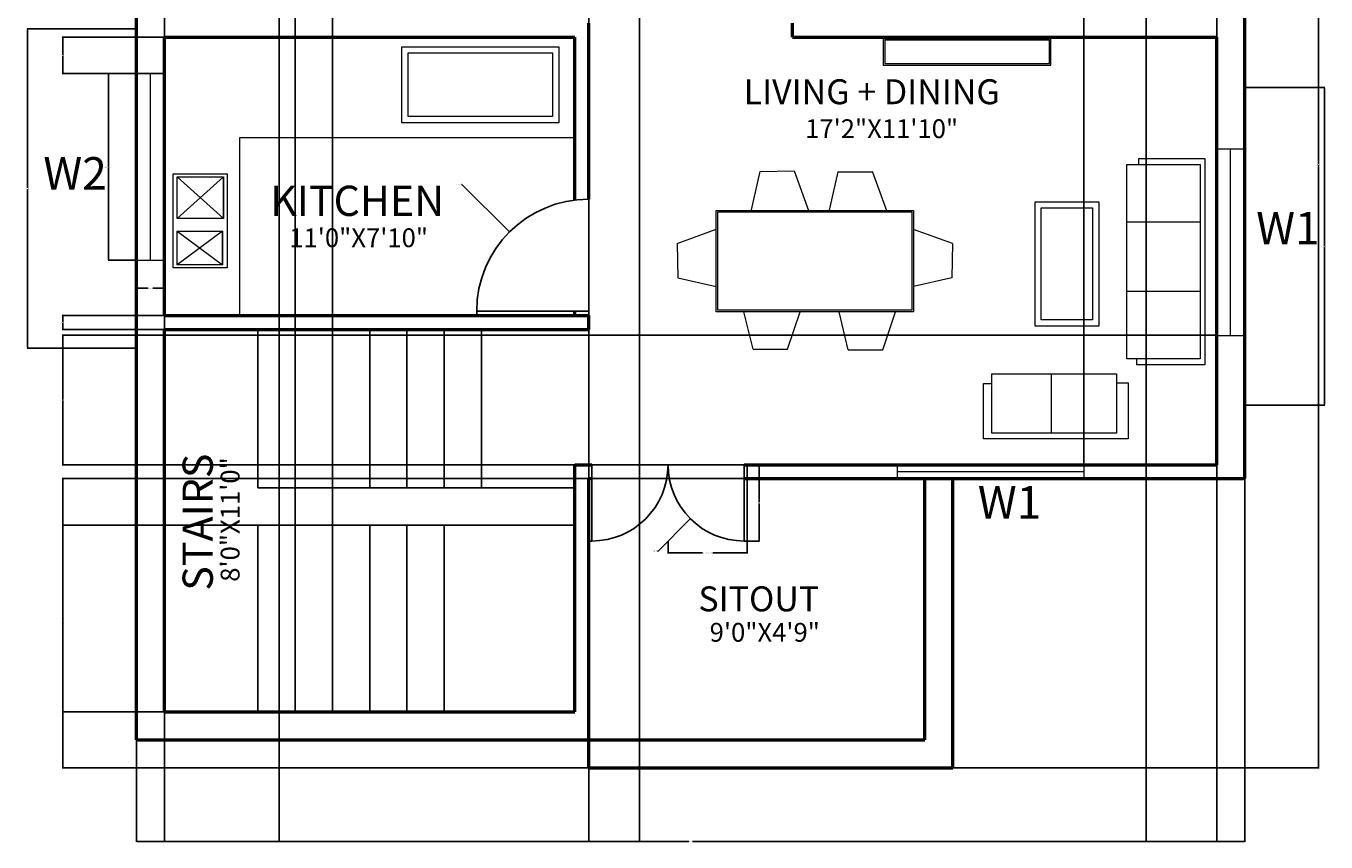
# Model space of a CAD drawing. Units: inches. Extents: x -26 to 394, y -29 to 465.
# Tile 1 of 2: x -26 to 392, y -29 to 234. Entities that reach past the tile are written whole.
import ezdxf

# ---------------------------------------------------------------- set-up
doc = ezdxf.new("R2010")
doc.units = ezdxf.units.IN
doc.header["$MEASUREMENT"] = 0
for name, color, linetype, lineweight, true_color in [('A-ANNO-DIMS', 254, 'Continuous', 18, 0xfeeab9), ('A-FLOR-FIXT', 254, 'Continuous', 18, 0xfeeab9), ('A-FURN', 254, 'Continuous', 18, 0xfeeab9)]:
    doc.layers.add(name, color=color, linetype=linetype, lineweight=lineweight, true_color=true_color)
for name, color, linetype, lineweight in [('A-ANNO-TEXT', 7, 'Continuous', 18), ('A-AREA-IDEN', 7, 'Continuous', 25), ('A-DOOR', 3, 'Continuous', 25), ('A-FLOR-STRS', 7, 'Continuous', 25), ('A-GLAZ', 4, 'Continuous', 18), ('A-WALL', 7, 'Continuous', 50)]:
    doc.layers.add(name, color=color, linetype=linetype, lineweight=lineweight)
doc.styles.get("Standard").update_dxf_attribs({"font": 'arial.ttf'})
doc.dimstyles.get("Standard").update_dxf_attribs({"dimtxt": 0.18, "dimasz": 0.18, "dimexe": 0.18, "dimexo": 0.0625, "dimgap": 0.09, "dimtad": 0, "dimtih": 1, "dimtoh": 1, "dimdec": 4, "dimzin": 0, "dimdsep": 46, "dimtxsty": 'Standard', "dimcen": 0.09, "dimadec": 0, "dimazin": 0, "dimtfac": 1, "dimtdec": 4, "dimtofl": 0, "dimtmove": 0, "dimatfit": 3, "dimfxl": 1, "dimtolj": 1, "dimtzin": 0, "dimarcsym": 0})

# ---------------------------------------------------------------- blocks, each defined once
blk = doc.blocks.new('*D10')
at = {"layer": 'A-ANNO-DIMS', "color": 0, "lineweight": -2, "transparency": 16777216}
for p, q in [((366.09, 214), (392.09, 214)), ((391.91, 213.82), (391.91, 163.15)), ((391.91, 112.11), (391.91, 162.79)), ((366.09, 111.93), (392.09, 111.93))]:
    blk.add_line(p, q, dxfattribs=at)
at = {"layer": 'A-ANNO-DIMS', "color": 0, "transparency": 16777216}
for points in [[(391.88, 213.82), (391.94, 213.82), (391.91, 214)], [(391.88, 112.11), (391.94, 112.11), (391.91, 111.93)]]:
    blk.add_solid(points, dxfattribs=at)
at = {"layer": 'Defpoints', "color": 0, "transparency": 16777216}
for p in [(366.02, 214), (366.02, 111.93), (391.91, 111.93)]:
    blk.add_point(p, dxfattribs=at)
at = {"layer": 'A-ANNO-DIMS', "color": 0, "transparency": 16777216, "insert": (391.91, 162.97), "char_height": 0.18, "attachment_point": 5}
blk.add_mtext('\\A1;102.0697', dxfattribs=at)
blk = doc.blocks.new('*D11')
at = {"layer": 'A-ANNO-DIMS', "color": 0, "lineweight": -2, "transparency": 16777216}
for p, q in [((9.7, 232.88), (-25.34, 232.88)), ((-25.16, 232.7), (-25.16, 181.74)), ((-25.16, 130.42), (-25.16, 181.38)), ((9.7, 130.24), (-25.34, 130.24))]:
    blk.add_line(p, q, dxfattribs=at)
at = {"layer": 'A-ANNO-DIMS', "color": 0, "transparency": 16777216}
for points in [[(-25.19, 232.7), (-25.13, 232.7), (-25.16, 232.88)], [(-25.19, 130.42), (-25.13, 130.42), (-25.16, 130.24)]]:
    blk.add_solid(points, dxfattribs=at)
at = {"layer": 'Defpoints', "color": 0, "transparency": 16777216}
for p in [(9.77, 232.88), (-25.16, 130.24), (9.77, 130.24)]:
    blk.add_point(p, dxfattribs=at)
at = {"layer": 'A-ANNO-DIMS', "color": 0, "transparency": 16777216, "insert": (-25.16, 181.56), "char_height": 0.18, "attachment_point": 5}
blk.add_mtext('\\A1;102.6356', dxfattribs=at)
blk = doc.blocks.new('WIN-60IN-9IN-JAMB')
for p, q in [((0, 9), (0, 0)), ((60, 9), (60, 0)), ((0, 4.5), (60, 4.5))]:
    blk.add_line(p, q)
blk = doc.blocks.new('DOOR-36IN-INTERIOR')
blk.add_lwpolyline([(0, 1.36), (0, 0), (36.04, 0), (36.04, 1.36)], close=True)
blk.add_arc((36, 1.36), 36, 90, 180)
blk = doc.blocks.new('DOOR-ENTRY-LEAF')
blk.add_lwpolyline([(24.53, 0), (25.46, 0), (25.46, 24.56), (24.53, 24.56)], close=True)
blk.add_arc((24.53, 24.53), 24.53, 180, 270)
blk = doc.blocks.new('FURN-WALL-UNIT')
for points in [[(8.48, 53.93), (0, 53.93), (0, 0), (8.48, 0)], [(7.98, 53.43), (0.5, 53.43), (0.5, 0.5), (7.98, 0.5)]]:
    blk.add_lwpolyline(points, close=True)
blk = doc.blocks.new('*D18')
at = {"layer": 'A-ANNO-DIMS', "color": 0, "lineweight": -2, "transparency": 16777216}
for p, q in [((9.84, 218.5), (0.72, 218.5)), ((0.9, 218.32), (0.9, 188.68)), ((0.9, 158.68), (0.9, 188.32)), ((9.84, 158.5), (0.72, 158.5))]:
    blk.add_line(p, q, dxfattribs=at)
at = {"layer": 'A-ANNO-DIMS', "color": 0, "transparency": 16777216}
for points in [[(0.87, 218.32), (0.93, 218.32), (0.9, 218.5)], [(0.87, 158.68), (0.93, 158.68), (0.9, 158.5)]]:
    blk.add_solid(points, dxfattribs=at)
at = {"layer": 'Defpoints', "color": 0, "transparency": 16777216}
for p in [(0.9, 218.5), (9.9, 218.5), (9.9, 158.5)]:
    blk.add_point(p, dxfattribs=at)
at = {"layer": 'A-ANNO-DIMS', "color": 0, "transparency": 16777216, "insert": (0.9, 188.5), "char_height": 0.18, "attachment_point": 5}
blk.add_mtext('\\A1;WINDOW 60.0000 TYP.', dxfattribs=at)
blk = doc.blocks.new('*D19')
at = {"layer": 'A-ANNO-DIMS', "color": 0, "lineweight": -2, "transparency": 16777216}
for p, q in [((9.9, 158.44), (9.9, 149.32)), ((18.9, 158.44), (18.9, 149.32)), ((10.08, 149.5), (13.63, 149.5)), ((18.72, 149.5), (15.17, 149.5))]:
    blk.add_line(p, q, dxfattribs=at)
at = {"layer": 'A-ANNO-DIMS', "color": 0, "transparency": 16777216}
for points in [[(10.08, 149.53), (10.08, 149.47), (9.9, 149.5)], [(18.72, 149.53), (18.72, 149.47), (18.9, 149.5)]]:
    blk.add_solid(points, dxfattribs=at)
at = {"layer": 'Defpoints', "color": 0, "transparency": 16777216}
for p in [(9.9, 158.5), (18.9, 158.5), (9.9, 149.5)]:
    blk.add_point(p, dxfattribs=at)
at = {"layer": 'A-ANNO-DIMS', "color": 0, "transparency": 16777216, "insert": (14.4, 149.5), "char_height": 0.18, "attachment_point": 5}
blk.add_mtext('\\A1;9.0000 TYP.', dxfattribs=at)
blk = doc.blocks.new('*D26')
at = {"layer": 'A-ANNO-DIMS', "color": 0, "lineweight": -2, "transparency": 16777216}
for p, q in [((180.81, 68.15), (180.81, 64.22)), ((206.27, 68.15), (206.27, 64.22)), ((180.99, 64.4), (191.89, 64.4)), ((206.09, 64.4), (195.19, 64.4))]:
    blk.add_line(p, q, dxfattribs=at)
at = {"layer": 'A-ANNO-DIMS', "color": 0, "transparency": 16777216}
for points in [[(180.99, 64.43), (180.99, 64.37), (180.81, 64.4)], [(206.09, 64.43), (206.09, 64.37), (206.27, 64.4)]]:
    blk.add_solid(points, dxfattribs=at)
at = {"layer": 'Defpoints', "color": 0, "transparency": 16777216}
for p in [(180.81, 68.21), (206.27, 68.21), (206.27, 64.4)]:
    blk.add_point(p, dxfattribs=at)
at = {"layer": 'A-ANNO-DIMS', "color": 0, "transparency": 16777216, "insert": (193.54, 64.4), "char_height": 0.18, "attachment_point": 5}
blk.add_mtext('\\A1;ENTRY LEAF 25.4567 TYP.', dxfattribs=at)
blk = doc.blocks.new('*D27')
at = {"layer": 'A-ANNO-DIMS', "color": 0, "lineweight": -2, "transparency": 16777216}
for p, q in [((206.33, 92.77), (210.27, 92.77)), ((210.09, 92.59), (210.09, 80.67)), ((210.09, 68.39), (210.09, 80.31)), ((206.33, 68.21), (210.27, 68.21))]:
    blk.add_line(p, q, dxfattribs=at)
at = {"layer": 'A-ANNO-DIMS', "color": 0, "transparency": 16777216}
for points in [[(210.06, 92.59), (210.12, 92.59), (210.09, 92.77)], [(210.06, 68.39), (210.12, 68.39), (210.09, 68.21)]]:
    blk.add_solid(points, dxfattribs=at)
at = {"layer": 'Defpoints', "color": 0, "transparency": 16777216}
for p in [(206.27, 92.77), (210.09, 92.77), (206.27, 68.21)]:
    blk.add_point(p, dxfattribs=at)
at = {"layer": 'A-ANNO-DIMS', "color": 0, "transparency": 16777216, "insert": (210.09, 80.49), "char_height": 0.18, "attachment_point": 5}
blk.add_mtext('\\A1;24.5570 TYP.', dxfattribs=at)
blk = doc.blocks.new('*D30')
at = {"layer": 'A-ANNO-DIMS', "color": 0, "lineweight": -2, "transparency": 16777216}
for p, q in [((366.35, 88.21), (366.35, -28.56)), ((9.85, 4.21), (9.85, -28.56)), ((10.03, -28.38), (187.5, -28.38)), ((366.17, -28.38), (188.71, -28.38))]:
    blk.add_line(p, q, dxfattribs=at)
at = {"layer": 'A-ANNO-DIMS', "color": 0, "transparency": 16777216}
for points in [[(10.03, -28.35), (10.03, -28.41), (9.85, -28.38)], [(366.17, -28.35), (366.17, -28.41), (366.35, -28.38)]]:
    blk.add_solid(points, dxfattribs=at)
at = {"layer": 'Defpoints', "color": 0, "transparency": 16777216}
for p in [(366.35, 88.27), (9.85, 4.27), (366.35, -28.38)]:
    blk.add_point(p, dxfattribs=at)
at = {"layer": 'A-ANNO-DIMS', "color": 0, "transparency": 16777216, "insert": (188.1, -28.38), "char_height": 0.18, "attachment_point": 5}
blk.add_mtext('\\A1;356.5000', dxfattribs=at)
blk = doc.blocks.new('*D31')
at = {"layer": 'A-ANNO-DIMS', "color": 0, "lineweight": -2, "transparency": 16777216}
for p, q in [((366.42, 383.27), (390.18, 383.27)), ((390, 383.09), (390, 189.45)), ((390, -4.55), (390, 189.09)), ((272.42, -4.73), (390.18, -4.73))]:
    blk.add_line(p, q, dxfattribs=at)
at = {"layer": 'A-ANNO-DIMS', "color": 0, "transparency": 16777216}
for points in [[(389.97, 383.09), (390.03, 383.09), (390, 383.27)], [(389.97, -4.55), (390.03, -4.55), (390, -4.73)]]:
    blk.add_solid(points, dxfattribs=at)
at = {"layer": 'Defpoints', "color": 0, "transparency": 16777216}
for p in [(366.35, 383.27), (390, 383.27), (272.35, -4.73)]:
    blk.add_point(p, dxfattribs=at)
at = {"layer": 'A-ANNO-DIMS', "color": 0, "transparency": 16777216, "insert": (390, 189.27), "char_height": 0.18, "attachment_point": 5}
blk.add_mtext('\\A1;388.0000', dxfattribs=at)
blk = doc.blocks.new('*D32')
at = {"layer": 'A-ANNO-DIMS', "color": 0, "lineweight": -2, "transparency": 16777216}
for p, q in [((272.29, 88.27), (-14.04, 88.27)), ((-13.86, 88.09), (-13.86, 41.95)), ((-13.86, -4.55), (-13.86, 41.59)), ((272.29, -4.73), (-14.04, -4.73))]:
    blk.add_line(p, q, dxfattribs=at)
at = {"layer": 'A-ANNO-DIMS', "color": 0, "transparency": 16777216}
for points in [[(-13.89, 88.09), (-13.83, 88.09), (-13.86, 88.27)], [(-13.89, -4.55), (-13.83, -4.55), (-13.86, -4.73)]]:
    blk.add_solid(points, dxfattribs=at)
at = {"layer": 'Defpoints', "color": 0, "transparency": 16777216}
for p in [(-13.86, 88.27), (272.35, 88.27), (272.35, -4.73)]:
    blk.add_point(p, dxfattribs=at)
at = {"layer": 'A-ANNO-DIMS', "color": 0, "transparency": 16777216, "insert": (-13.86, 41.77), "char_height": 0.18, "attachment_point": 5}
blk.add_mtext('\\A1;93.0000', dxfattribs=at)
blk = doc.blocks.new('*D34')
at = {"layer": 'A-ANNO-DIMS', "color": 0, "lineweight": -2, "transparency": 16777216}
for p, q in [((155.35, 374.21), (155.35, -28.56)), ((171.67, 374.21), (171.67, -28.56)), ((155.53, -28.38), (162.99, -28.38)), ((171.49, -28.38), (164.04, -28.38))]:
    blk.add_line(p, q, dxfattribs=at)
at = {"layer": 'A-ANNO-DIMS', "color": 0, "transparency": 16777216}
for points in [[(155.53, -28.35), (155.53, -28.41), (155.35, -28.38)], [(171.49, -28.35), (171.49, -28.41), (171.67, -28.38)]]:
    blk.add_solid(points, dxfattribs=at)
at = {"layer": 'Defpoints', "color": 0, "transparency": 16777216}
for p in [(155.35, 374.27), (171.67, 374.27), (171.67, -28.38)]:
    blk.add_point(p, dxfattribs=at)
at = {"layer": 'A-ANNO-DIMS', "color": 0, "transparency": 16777216, "insert": (163.51, -28.38), "char_height": 0.18, "attachment_point": 5}
blk.add_mtext('\\A1;16.3118', dxfattribs=at)
blk = doc.blocks.new('*D35')
at = {"layer": 'A-ANNO-DIMS', "color": 0, "lineweight": -2, "transparency": 16777216}
for p, q in [((314.49, 92.86), (314.49, 407.1)), ((314.67, 406.92), (335.38, 406.92)), ((357.17, 406.92), (336.46, 406.92)), ((357.35, 92.83), (357.35, 407.1))]:
    blk.add_line(p, q, dxfattribs=at)
at = {"layer": 'A-ANNO-DIMS', "color": 0, "transparency": 16777216}
for points in [[(314.67, 406.95), (314.67, 406.89), (314.49, 406.92)], [(357.17, 406.95), (357.17, 406.89), (357.35, 406.92)]]:
    blk.add_solid(points, dxfattribs=at)
at = {"layer": 'Defpoints', "color": 0, "transparency": 16777216}
for p in [(357.35, 406.92), (314.49, 92.8), (357.35, 92.77)]:
    blk.add_point(p, dxfattribs=at)
at = {"layer": 'A-ANNO-DIMS', "color": 0, "transparency": 16777216, "insert": (335.92, 406.92), "char_height": 0.18, "attachment_point": 5}
blk.add_mtext('\\A1;42.8686', dxfattribs=at)
blk = doc.blocks.new('*D36')
at = {"layer": 'A-ANNO-DIMS', "color": 0, "lineweight": -2, "transparency": 16777216}
for p, q in [((18.85, 374.21), (18.85, -28.56)), ((55.78, 374.2), (55.78, -28.56)), ((19.03, -28.38), (36.78, -28.38)), ((55.6, -28.38), (37.85, -28.38))]:
    blk.add_line(p, q, dxfattribs=at)
at = {"layer": 'A-ANNO-DIMS', "color": 0, "transparency": 16777216}
for points in [[(19.03, -28.35), (19.03, -28.41), (18.85, -28.38)], [(55.6, -28.35), (55.6, -28.41), (55.78, -28.38)]]:
    blk.add_solid(points, dxfattribs=at)
at = {"layer": 'Defpoints', "color": 0, "transparency": 16777216}
for p in [(18.85, 374.27), (55.78, 374.27), (55.78, -28.38)]:
    blk.add_point(p, dxfattribs=at)
at = {"layer": 'A-ANNO-DIMS', "color": 0, "transparency": 16777216, "insert": (37.31, -28.38), "char_height": 0.18, "attachment_point": 5}
blk.add_mtext('\\A1;36.9207', dxfattribs=at)
blk = doc.blocks.new('*D37')
at = {"layer": 'A-ANNO-DIMS', "color": 0, "lineweight": -2, "transparency": 16777216}
for p, q in [((334.57, 374.05), (334.57, -28.56)), ((357.35, 374.21), (357.35, -28.56)), ((334.75, -28.38), (345.43, -28.38)), ((357.17, -28.38), (346.5, -28.38))]:
    blk.add_line(p, q, dxfattribs=at)
at = {"layer": 'A-ANNO-DIMS', "color": 0, "transparency": 16777216}
for points in [[(334.75, -28.35), (334.75, -28.41), (334.57, -28.38)], [(357.17, -28.35), (357.17, -28.41), (357.35, -28.38)]]:
    blk.add_solid(points, dxfattribs=at)
at = {"layer": 'Defpoints', "color": 0, "transparency": 16777216}
for p in [(334.57, 374.11), (357.35, 374.27), (357.35, -28.38)]:
    blk.add_point(p, dxfattribs=at)
at = {"layer": 'A-ANNO-DIMS', "color": 0, "transparency": 16777216, "insert": (345.96, -28.38), "char_height": 0.18, "attachment_point": 5}
blk.add_mtext('\\A1;22.7852', dxfattribs=at)
blk = doc.blocks.new('*D39')
at = {"layer": 'A-ANNO-DIMS', "color": 0, "lineweight": -2, "transparency": 16777216}
for p, q in [((18.79, 230.27), (-14.04, 230.27)), ((-13.86, 230.09), (-13.86, 224.57)), ((-13.86, 218.68), (-13.86, 224.2)), ((18.84, 218.5), (-14.04, 218.5))]:
    blk.add_line(p, q, dxfattribs=at)
at = {"layer": 'A-ANNO-DIMS', "color": 0, "transparency": 16777216}
for points in [[(-13.89, 230.09), (-13.83, 230.09), (-13.86, 230.27)], [(-13.89, 218.68), (-13.83, 218.68), (-13.86, 218.5)]]:
    blk.add_solid(points, dxfattribs=at)
at = {"layer": 'Defpoints', "color": 0, "transparency": 16777216}
for p in [(18.85, 230.27), (-13.86, 218.5), (18.9, 218.5)]:
    blk.add_point(p, dxfattribs=at)
at = {"layer": 'A-ANNO-DIMS', "color": 0, "transparency": 16777216, "insert": (-13.86, 224.39), "char_height": 0.18, "attachment_point": 5}
blk.add_mtext('\\A1;11.7710', dxfattribs=at)
blk = doc.blocks.new('*D41')
at = {"layer": 'A-ANNO-DIMS', "color": 0, "lineweight": -2, "transparency": 16777216}
for p, q in [((357.17, 134.36), (-14.04, 134.36)), ((-13.86, 134.18), (-13.86, 113.75)), ((-13.86, 92.95), (-13.86, 113.38)), ((357.29, 92.77), (-14.04, 92.77))]:
    blk.add_line(p, q, dxfattribs=at)
at = {"layer": 'A-ANNO-DIMS', "color": 0, "transparency": 16777216}
for points in [[(-13.89, 134.18), (-13.83, 134.18), (-13.86, 134.36)], [(-13.89, 92.95), (-13.83, 92.95), (-13.86, 92.77)]]:
    blk.add_solid(points, dxfattribs=at)
at = {"layer": 'Defpoints', "color": 0, "transparency": 16777216}
for p in [(-13.86, 134.36), (357.24, 134.36), (357.35, 92.77)]:
    blk.add_point(p, dxfattribs=at)
at = {"layer": 'A-ANNO-DIMS', "color": 0, "transparency": 16777216, "insert": (-13.86, 113.56), "char_height": 0.18, "attachment_point": 5}
blk.add_mtext('\\A1;41.5853', dxfattribs=at)
blk = doc.blocks.new('*D42')
at = {"layer": 'A-ANNO-DIMS', "color": 0, "lineweight": -2, "transparency": 16777216}
for p, q in [((60.85, 73.33), (60.85, 407.1)), ((61.03, 406.92), (66.33, 406.92)), ((72.67, 406.92), (67.38, 406.92)), ((72.85, 73.33), (72.85, 407.1))]:
    blk.add_line(p, q, dxfattribs=at)
at = {"layer": 'A-ANNO-DIMS', "color": 0, "transparency": 16777216}
for points in [[(61.03, 406.95), (61.03, 406.89), (60.85, 406.92)], [(72.67, 406.95), (72.67, 406.89), (72.85, 406.92)]]:
    blk.add_solid(points, dxfattribs=at)
at = {"layer": 'Defpoints', "color": 0, "transparency": 16777216}
for p in [(72.85, 406.92), (60.85, 73.27), (72.85, 73.27)]:
    blk.add_point(p, dxfattribs=at)
at = {"layer": 'A-ANNO-DIMS', "color": 0, "transparency": 16777216, "insert": (66.85, 406.92), "char_height": 0.18, "attachment_point": 5}
blk.add_mtext('\\A1;12.0000', dxfattribs=at)
blk = doc.blocks.new('*D43')
at = {"layer": 'A-ANNO-DIMS', "color": 0, "lineweight": -2, "transparency": 16777216}
for p, q in [((150.79, 73.27), (-14.04, 73.27)), ((-13.86, 73.09), (-13.86, 43.45)), ((-13.86, 13.45), (-13.86, 43.09)), ((150.79, 13.27), (-14.04, 13.27))]:
    blk.add_line(p, q, dxfattribs=at)
at = {"layer": 'A-ANNO-DIMS', "color": 0, "transparency": 16777216}
for points in [[(-13.89, 73.09), (-13.83, 73.09), (-13.86, 73.27)], [(-13.89, 13.45), (-13.83, 13.45), (-13.86, 13.27)]]:
    blk.add_solid(points, dxfattribs=at)
at = {"layer": 'Defpoints', "color": 0, "transparency": 16777216}
for p in [(-13.86, 73.27), (150.85, 73.27), (150.85, 13.27)]:
    blk.add_point(p, dxfattribs=at)
at = {"layer": 'A-ANNO-DIMS', "color": 0, "transparency": 16777216, "insert": (-13.86, 43.27), "char_height": 0.18, "attachment_point": 5}
blk.add_mtext('\\A1;60.0000', dxfattribs=at)
blk = doc.blocks.new('*D44')
at = {"layer": 'A-ANNO-DIMS', "color": 0, "lineweight": -2, "transparency": 16777216}
for p, q in [((18.79, 140.77), (-14.04, 140.77)), ((-13.86, 140.59), (-13.86, 138.7)), ((-13.86, 136.45), (-13.86, 138.34)), ((18.79, 136.27), (-14.04, 136.27))]:
    blk.add_line(p, q, dxfattribs=at)
at = {"layer": 'A-ANNO-DIMS', "color": 0, "transparency": 16777216}
for points in [[(-13.89, 140.59), (-13.83, 140.59), (-13.86, 140.77)], [(-13.89, 136.45), (-13.83, 136.45), (-13.86, 136.27)]]:
    blk.add_solid(points, dxfattribs=at)
at = {"layer": 'Defpoints', "color": 0, "transparency": 16777216}
for p in [(-13.86, 140.77), (18.85, 140.77), (18.85, 136.27)]:
    blk.add_point(p, dxfattribs=at)
at = {"layer": 'A-ANNO-DIMS', "color": 0, "transparency": 16777216, "insert": (-13.86, 138.52), "char_height": 0.18, "attachment_point": 5}
blk.add_mtext('\\A1;4.5000', dxfattribs=at)
blk = doc.blocks.new('*D45')
at = {"layer": 'A-ANNO-DIMS', "color": 0, "lineweight": -2, "transparency": 16777216}
for p, q in [((114.36, 182.86), (114.54, 182.86)), ((114.54, 182.86), (129.69, 167.72)), ((155.27, 142.04), (155.27, 142.22)), ((155.18, 142.13), (155.36, 142.13))]:
    blk.add_line(p, q, dxfattribs=at)
at = {"layer": 'A-ANNO-DIMS', "color": 0, "transparency": 16777216}
blk.add_solid([(129.71, 167.74), (129.67, 167.7), (129.81, 167.59)], dxfattribs=at)
at = {"layer": 'Defpoints', "color": 0, "transparency": 16777216}
for p in [(129.81, 167.59), (155.27, 142.13)]:
    blk.add_point(p, dxfattribs=at)
at = {"layer": 'A-ANNO-DIMS', "color": 0, "transparency": 16777216, "insert": (113.54, 182.86), "char_height": 0.18, "attachment_point": 5}
blk.add_mtext('\\A1;4X R36.0000', dxfattribs=at)
blk = doc.blocks.new('*D46')
at = {"layer": 'A-ANNO-DIMS', "color": 0, "lineweight": -2, "transparency": 16777216}
for p, q in [((205.25, 92.74), (205.43, 92.74)), ((205.34, 92.65), (205.34, 92.83)), ((177.59, 64.99), (187.87, 75.27)), ((177.41, 64.99), (177.59, 64.99))]:
    blk.add_line(p, q, dxfattribs=at)
at = {"layer": 'A-ANNO-DIMS', "color": 0, "transparency": 16777216}
blk.add_solid([(187.85, 75.29), (187.89, 75.25), (188, 75.4)], dxfattribs=at)
at = {"layer": 'Defpoints', "color": 0, "transparency": 16777216}
for p in [(205.34, 92.74), (188, 75.4)]:
    blk.add_point(p, dxfattribs=at)
at = {"layer": 'A-ANNO-DIMS', "color": 0, "transparency": 16777216, "insert": (176.59, 64.99), "char_height": 0.18, "attachment_point": 5}
blk.add_mtext('\\A1;2X R24.5283', dxfattribs=at)

msp = doc.modelspace()

# ---------------------------------------------------------------- linework, layer by layer
at = {"layer": 'A-FLOR-FIXT'}
for p, q in [((43.09834, 140.92714), (43.09834, 197.93992)), ((43.09834, 197.93992), (150.8905, 197.93992)), ((22.97076, 185.36801), (37.84676, 171.90484)), ((37.84676, 185.36801), (22.97076, 171.90484)), ((37.84676, 171.90484), (37.84676, 185.36801)), ((22.97076, 167.88335), (37.4968, 157.04288)), ((37.4968, 167.88335), (22.97076, 157.04288)), ((37.4968, 157.04288), (37.4968, 167.88335))]:
    msp.add_line(p, q, dxfattribs=at)
for points in [[(95.18623, 227.16286), (145.69546, 227.16286), (145.69546, 202.68955), (95.18623, 202.68955)], [(97.18623, 225.16286), (143.69546, 225.16286), (143.69546, 204.68955), (97.18623, 204.68955)], [(21.67127, 186.33062), (39.03207, 186.33062), (39.03207, 156.08909), (21.67127, 156.08909)], [(22.97076, 185.36801), (37.84676, 185.36801), (37.84676, 171.90484), (22.97076, 171.90484)], [(22.97076, 167.88335), (37.4968, 167.88335), (37.4968, 157.04288), (22.97076, 157.04288)]]:
    msp.add_lwpolyline(points, close=True, dxfattribs=at)
at = {"layer": 'A-FLOR-STRS'}
for p, q in [((48.85458, 85.27084), (48.85458, 136.27084)), ((60.85458, 85.27084), (60.85458, 136.27084)), ((72.85458, 85.27084), (72.85458, 136.27084)), ((84.85458, 85.27084), (84.85458, 136.27084)), ((84.85458, 85.27084), (84.85458, 136.27084)), ((96.85458, 85.27084), (96.85458, 136.27084)), ((96.85458, 85.27084), (96.85458, 136.27084)), ((108.85458, 85.27084), (108.85458, 136.27084)), ((120.85458, 85.27084), (120.85458, 136.27084)), ((48.85458, 85.27084), (150.85458, 85.27084)), ((48.85458, 73.27084), (150.85458, 73.27084)), ((48.85458, 13.27084), (48.85458, 73.27084)), ((60.85458, 13.27084), (60.85458, 73.27084)), ((72.85458, 13.27084), (72.85458, 73.27084)), ((84.85458, 13.27084), (84.85458, 73.27084)), ((96.85458, 13.27084), (96.85458, 73.27084)), ((108.85458, 13.27084), (108.85458, 73.27084))]:
    msp.add_line(p, q, dxfattribs=at)
at = {"layer": 'A-FURN'}
for p, q in [((332.20912, 189.22649), (332.20912, 191.24443)), ((332.20912, 191.24443), (353.49512, 191.24443)), ((353.49512, 191.24443), (353.49512, 124.88737)), ((210.28735, 187.01727), (207.5651, 174.67281)), ((210.28735, 187.01727), (221.37704, 187.23708)), ((221.37704, 187.23708), (225.93246, 174.53943)), ((235.40598, 186.97999), (232.68374, 174.63554)), ((235.40598, 186.97999), (246.57454, 186.97999)), ((246.49568, 187.19981), (251.03772, 174.53943)), ((183.69841, 163.92246), (196.31887, 168.45018)), ((272.25398, 163.92246), (259.70233, 168.4255)), ((328.40123, 170.84579), (351.96728, 170.84579)), ((183.69841, 163.92246), (183.91823, 152.83277)), ((272.25398, 163.92246), (272.03417, 152.83277)), ((183.91823, 152.83277), (196.26268, 150.11052)), ((272.03417, 152.83277), (259.70233, 150.11331)), ((328.40123, 148.58145), (351.96728, 148.58145)), ((208.15692, 129.8587), (205.23898, 141.94626)), ((219.2488, 129.8587), (223.31681, 141.94626)), ((238.77166, 129.67882), (235.8103, 141.94626)), ((249.86353, 129.67882), (253.99141, 141.94424)), ((208.15692, 129.8587), (219.2488, 129.8587)), ((238.77166, 129.67882), (249.86353, 129.67882)), ((331.57406, 124.88737), (331.57406, 126.76561)), ((304.07407, 122.00747), (304.07407, 102.91906)), ((353.49512, 124.88737), (331.57406, 124.88737)), ((282.26785, 101.0517), (282.26785, 118.89522)), ((282.26785, 118.89522), (284.96781, 118.89522)), ((325.04955, 119.10272), (328.78781, 119.10272)), ((328.78781, 119.10272), (328.78781, 101.0517)), ((328.78781, 101.0517), (282.26785, 101.0517))]:
    msp.add_line(p, q, dxfattribs=at)
for points in [[(328.39018, 189.23927), (351.96018, 189.23927), (351.96018, 126.75875), (328.39018, 126.75875)], [(298.85104, 177.33318), (319.3576, 177.33318), (319.3576, 137.29006), (298.85104, 137.29006)], [(196.31887, 174.53943), (259.70233, 174.53943), (259.70233, 141.94626), (196.31887, 141.94626)], [(196.81887, 174.03943), (259.20233, 174.03943), (259.20233, 142.44626), (196.81887, 142.44626)], [(300.85104, 175.33318), (317.3576, 175.33318), (317.3576, 139.29006), (300.85104, 139.29006)], [(284.96781, 122.00747), (325.04955, 122.00747), (325.04955, 102.91906), (284.96781, 102.91906)]]:
    msp.add_lwpolyline(points, close=True, dxfattribs=at)
at = {"layer": 'A-GLAZ'}
for p, q in [((254.48603, 92.79767), (254.48603, 88.29767)), ((314.48603, 92.79767), (314.48603, 88.29767)), ((254.48603, 90.54767), (314.48603, 90.54767))]:
    msp.add_line(p, q, dxfattribs=at)
at = {"layer": 'A-WALL'}
for p, q in [((9.85458, 4.27084), (9.85458, 383.27084)), ((366.35458, 88.27084), (366.35458, 383.27084)), ((155.35458, 230.27084), (155.35458, 234.77084)), ((220.85458, 230.27084), (220.85458, 234.77084)), ((18.85458, 230.27084), (150.85458, 230.27084)), ((18.85458, 140.77084), (18.85458, 230.27084)), ((150.85458, 177.86169), (150.85458, 230.27084)), ((155.35458, 178.13342), (155.35458, 230.27084)), ((220.85458, 230.27084), (357.35458, 230.27084)), ((357.35458, 92.77084), (357.35458, 230.27084)), ((18.85458, 140.77084), (155.31243, 140.77084)), ((150.85458, 140.77084), (150.85458, 142.13352)), ((155.35458, 136.27084), (155.35458, 140.77084)), ((18.85458, 13.27084), (18.85458, 136.27084)), ((18.85458, 136.27084), (155.27027, 136.27084)), ((150.85458, 92.74212), (150.85458, 92.77084)), ((150.85458, 13.27084), (150.85458, 92.74212)), ((150.85458, 92.74212), (156.28304, 92.74212)), ((155.31243, 92.77084), (156.28304, 92.77084)), ((205.33961, 92.77084), (357.35458, 92.77084)), ((155.35458, -4.72916), (155.35458, 88.27084)), ((155.35458, 88.27084), (156.28304, 88.27084)), ((205.25259, 88.27084), (366.35458, 88.27084)), ((263.35458, 4.27084), (263.35458, 88.27084)), ((272.35458, -4.72916), (272.35458, 88.27084)), ((18.85458, 13.27084), (150.85458, 13.27084)), ((9.85458, 4.27084), (263.35458, 4.27084)), ((155.35458, -4.72916), (272.35458, -4.72916))]:
    msp.add_line(p, q, dxfattribs=at)

# ---------------------------------------------------------------- block references
at = {"layer": 'A-DOOR'}
for name, p in [('DOOR-36IN-INTERIOR', (119.27027, 140.77084)), ('DOOR-ENTRY-LEAF', (180.81132, 68.21383))]:
    msp.add_blockref(name, p, dxfattribs=at)
at = {"layer": 'A-DOOR', "extrusion": (0, 0, -1), "zscale": -1}
msp.add_blockref('DOOR-ENTRY-LEAF', (-180.81132, 68.21383), dxfattribs=at)
at = {"layer": 'A-FURN', "rotation": 270}
msp.add_blockref('FURN-WALL-UNIT', (250.037, 229.72497), dxfattribs=at)
at = {"layer": 'A-GLAZ', "rotation": 90.0000000000001}
for p in [(18.8992, 158.49982), (366.23608, 134.35612)]:
    msp.add_blockref('WIN-60IN-9IN-JAMB', p, dxfattribs=at)

# ---------------------------------------------------------------- texts
at = {"layer": 'A-ANNO-TEXT'}
for s, p in [('W2', (-20.09509, 181.23852)), ('W1', (369.96821, 163.61369)), ('W1', (280.44282, 75.44298))]:
    msp.add_text(s, height=10.431092, dxfattribs=at).set_placement(p)
at = {"layer": 'A-AREA-IDEN'}
for s, height, p in [('LIVING + DINING', 8.0236409, (205.12029, 208.67294)), ('17\'2"X11\'10"', 6.0480693, (224.9022, 197.77673)), ('KITCHEN', 9.719051, (52.85804, 172.75261)), ('11\'0"X7\'10"', 6.0480693, (58.99911, 162.70783)), ('SITOUT', 8.023641, (190.57098, 45.60842)), ('9\'0"X4\'9"', 6.048069, (194.19853, 35.83589))]:
    msp.add_text(s, height=height, dxfattribs=at).set_placement(p)
for s, height, p in [('STAIRS', 9.719051, (34.40884, 52.22652)), ('8\'0"X11\'0"', 6.048069, (42.9982, 55.11294))]:
    msp.add_text(s, height=height, rotation=90, dxfattribs=at).set_placement(p)

# ---------------------------------------------------------------- dimensions: what is measured, and where the dimension line sits
at = {"layer": 'A-ANNO-DIMS'}
for base, p1, p2, picture, middle in [((72.85458, 406.92148), (60.85458, 73.27084), (72.85458, 73.27084), '*D42', (66.85459, 406.92148)), ((357.354585, 406.921485), (314.486028, 92.797666), (357.354585, 92.770839), '*D35', (335.920306, 406.921485)), ((55.77527, -28.37916), (18.85458, 374.27084), (55.77527, 374.26724), '*D36', (37.31493, -28.37916)), ((171.66634, -28.37916), (155.35458, 374.27084), (171.66634, 374.27148), '*D34', (163.51046, -28.37916)), ((357.35458, -28.37916), (334.56939, 374.11204), (357.35458, 374.27084), '*D37', (345.96199, -28.37916)), ((366.35458, -28.37916), (9.85458, 4.27084), (366.35458, 88.27084), '*D30', (188.10458, -28.37916))]:
    dim = msp.add_linear_dim(base=base, p1=p1, p2=p2, dimstyle='Standard', override={"dimdec": 4, "dimlfac": 1, "dimrnd": 0, "dimzin": 0, "dimdsep": 46, "dimlunit": 2}, dxfattribs=at)
    dim.commit()
    dim.dimension.update_dxf_attribs({"geometry": picture, "text_midpoint": middle})
for base, p1, p2, override, picture, middle in [((390.00459, 383.27084), (272.35458, -4.72916), (366.35458, 383.27084), {"dimdec": 4, "dimlfac": 1, "dimrnd": 0, "dimzin": 0, "dimdsep": 46, "dimlunit": 2}, '*D31', (390.00459, 189.27084)), ((-25.16151, 130.24033), (9.76748, 232.87592), (9.76748, 130.24033), {"dimclrd": 0, "dimclre": 0, "dimclrt": 0}, '*D11', (-25.16151, 181.55813)), ((-13.85972, 218.49982), (18.85458, 230.27084), (18.8992, 218.49982), {"dimdec": 4, "dimlfac": 1, "dimrnd": 0, "dimzin": 0, "dimdsep": 46, "dimlunit": 2}, '*D39', (-13.85972, 224.38533)), ((391.90663, 111.93229), (366.02473, 214.00199), (366.02473, 111.93229), {"dimclrd": 0, "dimclre": 0, "dimclrt": 0}, '*D10', (391.90663, 162.96714)), ((-13.85972, 140.77084), (18.85458, 136.27084), (18.85458, 140.77084), {"dimdec": 4, "dimlfac": 1, "dimrnd": 0, "dimzin": 0, "dimdsep": 46, "dimlunit": 2}, '*D44', (-13.85972, 138.52084)), ((-13.85972, 134.35612), (357.35458, 92.77084), (357.23608, 134.35612), {"dimdec": 4, "dimlfac": 1, "dimrnd": 0, "dimzin": 0, "dimdsep": 46, "dimlunit": 2}, '*D41', (-13.85972, 113.56348)), ((-13.85972, 88.27084), (272.35458, -4.72916), (272.35458, 88.27084), {"dimdec": 4, "dimlfac": 1, "dimrnd": 0, "dimzin": 0, "dimdsep": 46, "dimlunit": 2}, '*D32', (-13.85972, 41.77084)), ((-13.85972, 73.27084), (150.85458, 13.27084), (150.85458, 73.27084), {"dimdec": 4, "dimlfac": 1, "dimrnd": 0, "dimzin": 0, "dimdsep": 46, "dimlunit": 2}, '*D43', (-13.85972, 43.27084))]:
    dim = msp.add_linear_dim(base=base, p1=p1, p2=p2, angle=90, dimstyle='Standard', override=override, dxfattribs=at)
    dim.commit()
    dim.dimension.update_dxf_attribs({"geometry": picture, "text_midpoint": middle})
for base, p1, p2, angle, text, picture, middle in [((0.8992, 218.49982), (9.8992, 158.49982), (9.8992, 218.49982), 90, 'WINDOW <> TYP.', '*D18', (0.8992, 188.49982)), ((9.8992, 149.49982), (18.8992, 158.49982), (9.8992, 158.49982), 180, '<> TYP.', '*D19', (14.3992, 149.49982)), ((210.08657, 92.77084), (206.26806, 68.21383), (206.26806, 92.77084), 90, '<> TYP.', '*D27', (210.08657, 80.49233))]:
    dim = msp.add_linear_dim(base=base, p1=p1, p2=p2, angle=angle, text=text, dimstyle='Standard', override={"dimdec": 4, "dimlfac": 1, "dimrnd": 0, "dimzin": 0, "dimdsep": 46, "dimlunit": 2}, dxfattribs=at)
    dim.commit()
    dim.dimension.update_dxf_attribs({"geometry": picture, "text_midpoint": middle})
for center, mpoint, text, picture, middle in [((155.27027, 142.13352), (129.81403, 167.58897), '4X <>', '*D45', (113.5439, 182.86224)), ((205.33961, 92.74212), (187.99525, 75.39825), '2X <>', '*D46', (176.59402, 64.99192))]:
    dim = msp.add_radius_dim(center=center, mpoint=mpoint, text=text, dimstyle='Standard', override={"dimdec": 4, "dimlfac": 1, "dimrnd": 0, "dimzin": 0, "dimdsep": 46, "dimlunit": 2}, dxfattribs=at)
    dim.commit()
    dim.dimension.update_dxf_attribs({"geometry": picture, "text_midpoint": middle, "dimtype": 164})
dim = msp.add_linear_dim(base=(206.26806, 64.39532), p1=(180.81132, 68.21383), p2=(206.26806, 68.21383), text='ENTRY LEAF <> TYP.', dimstyle='Standard', override={"dimdec": 4, "dimlfac": 1, "dimrnd": 0, "dimzin": 0, "dimdsep": 46, "dimlunit": 2}, dxfattribs=at)
dim.commit()
dim.dimension.update_dxf_attribs({"geometry": '*D26', "text_midpoint": (193.53969, 64.39532)})

doc.saveas('drawing.dxf')
